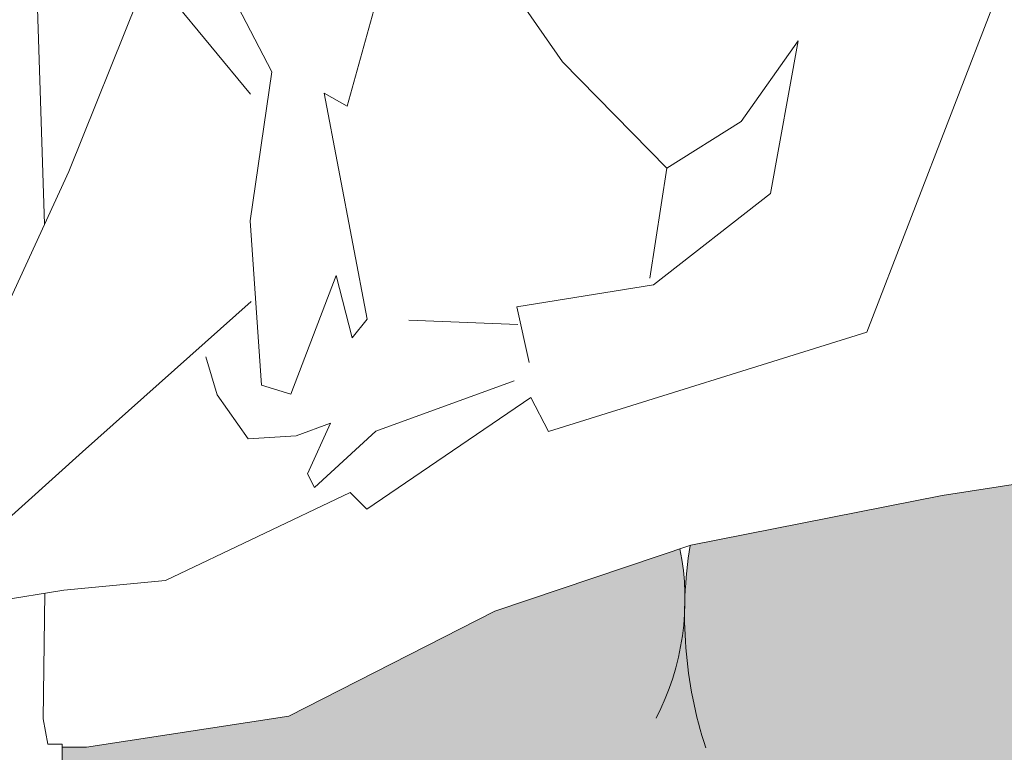
# Model space of a CAD drawing. Units: inches. Extents: x 1994 to 3075, y 3517 to 3950.
# Tile 35 of 58: x 1994.62882 to 1994.65094, y 3553.72103 to 3553.7375. Entities that reach past the tile are written whole.
import ezdxf

# ---------------------------------------------------------------- set-up
doc = ezdxf.new("R2010")
doc.units = ezdxf.units.IN
doc.layers.add('A-FURN-REFR', color=8, linetype='Continuous', lineweight=13)
doc.layers.add('A-FURN-REFR-PATT', color=8, linetype='Continuous', lineweight=13)

msp = doc.modelspace()

# ---------------------------------------------------------------- hatches: boundary and pattern name
at = {"layer": 'A-FURN-REFR-PATT'}
h = msp.add_hatch(color=256, dxfattribs=at)
h.set_gradient(color1=(238, 215, 180), color2=(243, 226, 201), one_color=1, tint=0.87)
edge = h.paths.add_edge_path()
edge.add_line((1994.681542, 3553.709525), (1994.682048, 3553.709217))
edge.add_line((1994.682048, 3553.709217), (1994.682631, 3553.708815))
edge.add_line((1994.682631, 3553.708815), (1994.682631, 3553.708383))
edge.add_line((1994.682631, 3553.708383), (1994.682498, 3553.704652))
edge.add_line((1994.682498, 3553.704652), (1994.682631, 3553.701474))
edge.add_line((1994.682631, 3553.701474), (1994.682631, 3553.700426))
edge.add_line((1994.682631, 3553.700426), (1994.682104, 3553.700396))
edge.add_line((1994.682104, 3553.700396), (1994.681598, 3553.699902))
edge.add_line((1994.681598, 3553.699902), (1994.681992, 3553.699717))
edge.add_line((1994.681992, 3553.699717), (1994.682631, 3553.699439))
edge.add_line((1994.682631, 3553.699439), (1994.682631, 3553.695334))
edge.add_ellipse((1994.680709, 3553.695334), major_axis=(0, 0.002111), ratio=0.910403, start_angle=180, end_angle=270, ccw=False)
edge.add_line((1994.680709, 3553.693223), (1994.680522, 3553.693223))
edge.add_line((1994.680522, 3553.693223), (1994.680314, 3553.694))
edge.add_ellipse((1994.68491, 3553.694998), major_axis=(0, 0.005146), ratio=0.910403, start_angle=92.3431, end_angle=102.2543, ccw=False)
edge.add_ellipse((1994.674568, 3553.694683), major_axis=(0, 0.006219), ratio=0.910403, start_angle=-88.7485, end_angle=-87.76)
edge.add_ellipse((1994.68491, 3553.694998), major_axis=(0, 0.005146), ratio=0.910403, start_angle=91.1484, end_angle=92.3431)
edge.add_ellipse((1994.674568, 3553.694683), major_axis=(0, 0.006219), ratio=0.910403, start_angle=262.8125, end_angle=271.2515, ccw=False)
edge.add_line((1994.680193, 3553.693973), (1994.679278, 3553.693223))
edge.add_line((1994.679278, 3553.693223), (1994.678042, 3553.693223))
edge.add_line((1994.678042, 3553.693223), (1994.673955, 3553.693055))
edge.add_line((1994.673955, 3553.693055), (1994.669892, 3553.693223))
edge.add_line((1994.669892, 3553.693223), (1994.669387, 3553.693223))
edge.add_line((1994.669387, 3553.693223), (1994.668536, 3553.693813))
edge.add_ellipse((1994.673095, 3553.694999), major_axis=(0, 0.005146), ratio=0.910403, start_angle=92.3431, end_angle=104.5922, ccw=False)
edge.add_ellipse((1994.662753, 3553.694684), major_axis=(0, 0.006219), ratio=0.910403, start_angle=-88.7485, end_angle=-87.76)
edge.add_ellipse((1994.673095, 3553.694999), major_axis=(0, 0.005146), ratio=0.910403, start_angle=91.1484, end_angle=92.3431)
edge.add_ellipse((1994.662753, 3553.694684), major_axis=(0, 0.006219), ratio=0.910403, start_angle=260.6759, end_angle=271.2515, ccw=False)
edge.add_line((1994.668352, 3553.693765), (1994.66822, 3553.693223))
edge.add_line((1994.66822, 3553.693223), (1994.666295, 3553.693223))
edge.add_line((1994.666295, 3553.693223), (1994.664702, 3553.693298))
edge.add_line((1994.664702, 3553.693298), (1994.660712, 3553.693051))
edge.add_line((1994.660712, 3553.693051), (1994.65764, 3553.693223))
edge.add_line((1994.65764, 3553.693223), (1994.656797, 3553.693223))
edge.add_line((1994.656797, 3553.693223), (1994.656116, 3553.693819))
edge.add_ellipse((1994.660616, 3553.695249), major_axis=(0, 0.005146), ratio=0.910403, start_angle=92.3431, end_angle=107.6246, ccw=False)
edge.add_ellipse((1994.650274, 3553.694934), major_axis=(0, 0.006219), ratio=0.910403, start_angle=-88.7485, end_angle=-87.76)
edge.add_ellipse((1994.660616, 3553.695249), major_axis=(0, 0.005146), ratio=0.910403, start_angle=91.1484, end_angle=92.3431)
edge.add_ellipse((1994.650274, 3553.694934), major_axis=(0, 0.006219), ratio=0.910403, start_angle=257.752, end_angle=271.2515, ccw=False)
edge.add_line((1994.655829, 3553.693728), (1994.654998, 3553.693223))
edge.add_line((1994.654998, 3553.693223), (1994.649752, 3553.692989))
edge.add_line((1994.649752, 3553.692989), (1994.644994, 3553.693223))
edge.add_line((1994.644994, 3553.693223), (1994.643952, 3553.693223))
edge.add_ellipse((1994.651853, 3553.695067), major_axis=(0, 0.008872), ratio=0.910403, start_angle=89.8354, end_angle=103.1369, ccw=False)
edge.add_ellipse((1994.638929, 3553.695405), major_axis=(0, 0.005332), ratio=0.910403, start_angle=266.2788, end_angle=270.7223)
edge.add_ellipse((1994.651853, 3553.695067), major_axis=(0, 0.008872), ratio=0.910403, start_angle=87.1651, end_angle=89.8354)
edge.add_ellipse((1994.638929, 3553.695405), major_axis=(0, 0.005332), ratio=0.910403, start_angle=243.7698, end_angle=266.2788, ccw=False)
edge.add_line((1994.643359, 3553.693223), (1994.642545, 3553.693223))
edge.add_line((1994.642545, 3553.693223), (1994.641153, 3553.693113))
edge.add_line((1994.641153, 3553.693113), (1994.636432, 3553.693359))
edge.add_line((1994.636432, 3553.693359), (1994.633777, 3553.693223))
edge.add_line((1994.633777, 3553.693223), (1994.63245, 3553.693223))
edge.add_line((1994.63245, 3553.693223), (1994.632375, 3553.693314))
edge.add_ellipse((1994.640193, 3553.695548), major_axis=(0, 0.008872), ratio=0.910403, start_angle=89.8354, end_angle=105.9456, ccw=False)
edge.add_ellipse((1994.627269, 3553.695886), major_axis=(0, 0.005332), ratio=0.910403, start_angle=266.2788, end_angle=270.7223)
edge.add_ellipse((1994.640193, 3553.695548), major_axis=(0, 0.008872), ratio=0.910403, start_angle=87.1651, end_angle=89.8354)
edge.add_ellipse((1994.627269, 3553.695886), major_axis=(0, 0.005332), ratio=0.910403, start_angle=237.8324, end_angle=266.2788, ccw=False)
edge.add_ellipse((1994.6317, 3553.695334), major_axis=(0, 0.002111), ratio=0.910403, start_angle=90, end_angle=174.0631, ccw=False)
edge.add_line((1994.629778, 3553.695334), (1994.629737, 3553.696763))
edge.add_line((1994.629737, 3553.696763), (1994.629778, 3553.698454))
edge.add_line((1994.629778, 3553.698454), (1994.629778, 3553.699441))
edge.add_line((1994.629778, 3553.699441), (1994.629962, 3553.700094))
edge.add_line((1994.629962, 3553.700094), (1994.630637, 3553.700403))
edge.add_line((1994.630637, 3553.700403), (1994.630075, 3553.700834))
edge.add_line((1994.630075, 3553.700834), (1994.629778, 3553.701292))
edge.add_line((1994.629778, 3553.701292), (1994.629778, 3553.702155))
edge.add_line((1994.629778, 3553.702155), (1994.630018, 3553.703363))
edge.add_line((1994.630018, 3553.703363), (1994.630018, 3553.706016))
edge.add_line((1994.630018, 3553.706016), (1994.629778, 3553.708015))
edge.add_line((1994.629778, 3553.708015), (1994.629778, 3553.70894))
edge.add_line((1994.629778, 3553.70894), (1994.630187, 3553.709347))
edge.add_line((1994.630187, 3553.709347), (1994.630918, 3553.70947))
edge.add_line((1994.630918, 3553.70947), (1994.630299, 3553.709902))
edge.add_line((1994.630299, 3553.709902), (1994.629778, 3553.710112))
edge.add_line((1994.629778, 3553.710112), (1994.629778, 3553.712086))
edge.add_line((1994.629778, 3553.712086), (1994.629962, 3553.713788))
edge.add_line((1994.629962, 3553.713788), (1994.629778, 3553.716158))
edge.add_line((1994.629778, 3553.716158), (1994.629778, 3553.718502))
edge.add_line((1994.629778, 3553.718502), (1994.630187, 3553.718908))
edge.add_line((1994.630187, 3553.718908), (1994.629778, 3553.719365))
edge.add_line((1994.629778, 3553.719365), (1994.629778, 3553.72115))
edge.add_line((1994.629778, 3553.72115), (1994.630322, 3553.72115))
edge.add_line((1994.630322, 3553.72115), (1994.634865, 3553.721849))
edge.add_line((1994.634865, 3553.721849), (1994.639494, 3553.724204))
edge.add_line((1994.639494, 3553.724204), (1994.643653, 3553.725608))
edge.add_ellipse((1994.63891, 3553.72447), major_axis=(0, 0.005332), ratio=0.910403, start_angle=270.7223, end_angle=283.4893, ccw=False)
edge.add_ellipse((1994.651833, 3553.724132), major_axis=(0, 0.008872), ratio=0.910403, start_angle=87.1651, end_angle=89.8354)
edge.add_ellipse((1994.63891, 3553.72447), major_axis=(0, 0.005332), ratio=0.910403, start_angle=266.2788, end_angle=270.7223)
edge.add_ellipse((1994.651833, 3553.724132), major_axis=(0, 0.008872), ratio=0.910403, start_angle=438.9501, end_angle=447.1651, ccw=False)
edge.add_line((1994.643881, 3553.725685), (1994.643897, 3553.72569))
edge.add_line((1994.643897, 3553.72569), (1994.649542, 3553.726806))
edge.add_line((1994.649542, 3553.726806), (1994.655977, 3553.727797))
edge.add_line((1994.655977, 3553.727797), (1994.658348, 3553.728382))
edge.add_ellipse((1994.662052, 3553.754177), major_axis=(0, 0.026115), ratio=0.910403, start_angle=171.8281, end_angle=180.2609)
edge.add_ellipse((1994.661314, 3553.682223), major_axis=(0, 0.04585), ratio=0.910403, start_angle=-1.0711, end_angle=-0.1044)
edge.add_ellipse((1994.662052, 3553.754177), major_axis=(0, 0.026115), ratio=0.910403, start_angle=171.8281, end_angle=178.5636, ccw=False)
edge.add_line((1994.658348, 3553.728382), (1994.666025, 3553.730275))
edge.add_line((1994.666025, 3553.730275), (1994.67483, 3553.732877))
edge.add_line((1994.67483, 3553.732877), (1994.680219, 3553.734687))
edge.add_ellipse((1994.675489, 3553.733489), major_axis=(0, 0.005332), ratio=0.910403, start_angle=270.7223, end_angle=284.2178, ccw=False)
edge.add_ellipse((1994.688412, 3553.73315), major_axis=(0, 0.008872), ratio=0.910403, start_angle=87.1651, end_angle=89.8354)
edge.add_ellipse((1994.675489, 3553.733489), major_axis=(0, 0.005332), ratio=0.910403, start_angle=266.2788, end_angle=270.7223)
edge.add_ellipse((1994.688412, 3553.73315), major_axis=(0, 0.008872), ratio=0.910403, start_angle=438.5005, end_angle=447.1651, ccw=False)
edge.add_line((1994.68047, 3553.734766), (1994.682205, 3553.735263))
edge.add_line((1994.682205, 3553.735263), (1994.682631, 3553.735263))
edge.add_line((1994.682631, 3553.735263), (1994.682631, 3553.734609))
edge.add_line((1994.682631, 3553.734609), (1994.682783, 3553.733623))
edge.add_line((1994.682783, 3553.733623), (1994.682631, 3553.730537))
edge.add_line((1994.682631, 3553.730537), (1994.682631, 3553.728749))
edge.add_line((1994.682631, 3553.728749), (1994.682334, 3553.728195))
edge.add_line((1994.682334, 3553.728195), (1994.681547, 3553.727824))
edge.add_line((1994.681547, 3553.727824), (1994.682053, 3553.727639))
edge.add_line((1994.682053, 3553.727639), (1994.682631, 3553.72733))
edge.add_line((1994.682631, 3553.72733), (1994.682631, 3553.725726))
edge.add_line((1994.682631, 3553.725726), (1994.682727, 3553.724308))
edge.add_line((1994.682727, 3553.724308), (1994.682631, 3553.721716))
edge.add_line((1994.682631, 3553.721716), (1994.682631, 3553.720165))
edge.add_line((1994.682631, 3553.720165), (1994.682329, 3553.719086))
edge.add_line((1994.682329, 3553.719086), (1994.681823, 3553.718654))
edge.add_line((1994.681823, 3553.718654), (1994.682329, 3553.718531))
edge.add_line((1994.682329, 3553.718531), (1994.682722, 3553.718346))
edge.add_line((1994.682722, 3553.718346), (1994.68261, 3553.715693))
edge.add_line((1994.68261, 3553.715693), (1994.682631, 3553.711159))
edge.add_line((1994.682631, 3553.711159), (1994.682631, 3553.710327))
edge.add_line((1994.682631, 3553.710327), (1994.682217, 3553.70971))
edge.add_line((1994.682217, 3553.70971), (1994.681542, 3553.709525))
edge = h.paths.add_edge_path(flags=16)
edge.add_ellipse((1994.674017, 3553.663488), major_axis=(0, 0.04585), ratio=0.910403, start_angle=-1.0711, end_angle=-0.1044)
edge.add_ellipse((1994.674755, 3553.735442), major_axis=(0, 0.026115), ratio=0.910403, start_angle=178.5636, end_angle=180.2609)
h.paths.add_polyline_path([(1994.668419, 3553.710039), (1994.668385, 3553.710026), (1994.668404, 3553.710013)], flags=16)
edge = h.paths.add_edge_path(flags=16)
edge.add_ellipse((1994.663397, 3553.714852), major_axis=(0, 0.005332), ratio=0.910403, start_angle=266.2788, end_angle=270.7223)
edge.add_ellipse((1994.67632, 3553.714514), major_axis=(0, 0.008872), ratio=0.910403, start_angle=87.1651, end_angle=89.8354)
edge = h.paths.add_edge_path(flags=16)
edge.add_ellipse((1994.662753, 3553.703926), major_axis=(0, 0.006219), ratio=0.910403, start_angle=-88.7485, end_angle=-87.76)
edge.add_ellipse((1994.673095, 3553.704241), major_axis=(0, 0.005146), ratio=0.910403, start_angle=91.1484, end_angle=92.3431)
h.paths.add_polyline_path([(1994.680357, 3553.710026), (1994.680376, 3553.710013), (1994.680391, 3553.710039)], flags=16)
edge = h.paths.add_edge_path(flags=16)
edge.add_ellipse((1994.684791, 3553.713857), major_axis=(0, 0.005146), ratio=0.910403, start_angle=91.1484, end_angle=92.3431)
edge.add_ellipse((1994.67445, 3553.713542), major_axis=(0, 0.006219), ratio=0.910403, start_angle=-88.7485, end_angle=-87.76)
h.paths.add_polyline_path([(1994.668404, 3553.719229), (1994.668419, 3553.719256), (1994.668385, 3553.719242)], flags=16)
edge = h.paths.add_edge_path(flags=16)
edge.add_ellipse((1994.68491, 3553.704625), major_axis=(0, 0.005146), ratio=0.910403, start_angle=91.1484, end_angle=92.3431)
edge.add_ellipse((1994.674568, 3553.70431), major_axis=(0, 0.006219), ratio=0.910403, start_angle=-88.7485, end_angle=-87.76)
edge = h.paths.add_edge_path(flags=16)
edge.add_ellipse((1994.662353, 3553.744655), major_axis=(0, 0.026115), ratio=0.910403, start_angle=178.5636, end_angle=180.2609)
edge.add_ellipse((1994.661615, 3553.6727), major_axis=(0, 0.04585), ratio=0.910403, start_angle=-1.0711, end_angle=-0.1044)
edge = h.paths.add_edge_path(flags=16)
edge.add_ellipse((1994.662621, 3553.722979), major_axis=(0, 0.006219), ratio=0.910403, start_angle=-88.7485, end_angle=-87.76)
edge.add_ellipse((1994.672963, 3553.723294), major_axis=(0, 0.005146), ratio=0.910403, start_angle=91.1484, end_angle=92.3431)
h.paths.add_polyline_path([(1994.68017, 3553.719242), (1994.680189, 3553.719229), (1994.680204, 3553.719256)], flags=16)
h.paths.add_polyline_path([(1994.668419, 3553.70036), (1994.668385, 3553.700347), (1994.668404, 3553.700334)], flags=16)
edge = h.paths.add_edge_path(flags=16)
edge.add_ellipse((1994.673942, 3553.654177), major_axis=(0, 0.04585), ratio=0.910403, start_angle=-1.0711, end_angle=-0.1044)
edge.add_ellipse((1994.67468, 3553.726132), major_axis=(0, 0.026115), ratio=0.910403, start_angle=178.5636, end_angle=180.2609)
edge = h.paths.add_edge_path(flags=16)
edge.add_ellipse((1994.685026, 3553.723294), major_axis=(0, 0.005146), ratio=0.910403, start_angle=91.1484, end_angle=92.3431)
edge.add_ellipse((1994.674684, 3553.722979), major_axis=(0, 0.006219), ratio=0.910403, start_angle=-88.7485, end_angle=-87.76)
h.paths.add_polyline_path([(1994.680569, 3553.70036), (1994.680535, 3553.700347), (1994.680554, 3553.700334)], flags=16)
h.paths.add_polyline_path([(1994.656068, 3553.710085), (1994.656034, 3553.710071), (1994.656052, 3553.710058)], flags=16)
h.paths.add_polyline_path([(1994.668404, 3553.728426), (1994.668419, 3553.728453), (1994.668385, 3553.728439)], flags=16)
edge = h.paths.add_edge_path(flags=16)
edge.add_ellipse((1994.650317, 3553.713896), major_axis=(0, 0.006219), ratio=0.910403, start_angle=-88.7485, end_angle=-87.76)
edge.add_ellipse((1994.660659, 3553.714211), major_axis=(0, 0.005146), ratio=0.910403, start_angle=91.1484, end_angle=92.3431)
edge = h.paths.add_edge_path(flags=16)
edge.add_ellipse((1994.650274, 3553.70431), major_axis=(0, 0.006219), ratio=0.910403, start_angle=-88.7485, end_angle=-87.76)
edge.add_ellipse((1994.660616, 3553.704625), major_axis=(0, 0.005146), ratio=0.910403, start_angle=91.1484, end_angle=92.3431)
h.paths.add_polyline_path([(1994.68033, 3553.728439), (1994.680349, 3553.728426), (1994.680364, 3553.728453)], flags=16)
h.paths.add_polyline_path([(1994.656052, 3553.719229), (1994.656068, 3553.719256), (1994.656034, 3553.719242)], flags=16)
edge = h.paths.add_edge_path(flags=16)
edge.add_ellipse((1994.649569, 3553.663672), major_axis=(0, 0.04585), ratio=0.910403, start_angle=-1.0711, end_angle=-0.1044)
edge.add_ellipse((1994.650307, 3553.735627), major_axis=(0, 0.026115), ratio=0.910403, start_angle=178.5636, end_angle=180.2609)
h.paths.add_polyline_path([(1994.656068, 3553.700324), (1994.656034, 3553.70031), (1994.656052, 3553.700297)], flags=16)
edge = h.paths.add_edge_path(flags=16)
edge.add_ellipse((1994.650446, 3553.723545), major_axis=(0, 0.006219), ratio=0.910403, start_angle=-88.7485, end_angle=-87.76)
edge.add_ellipse((1994.660788, 3553.72386), major_axis=(0, 0.005146), ratio=0.910403, start_angle=91.1484, end_angle=92.3431)
edge = h.paths.add_edge_path(flags=16)
edge.add_ellipse((1994.64966, 3553.654177), major_axis=(0, 0.04585), ratio=0.910403, start_angle=-1.0711, end_angle=-0.1044)
edge.add_ellipse((1994.650398, 3553.726132), major_axis=(0, 0.026115), ratio=0.910403, start_angle=178.5636, end_angle=180.2609)
h.paths.add_polyline_path([(1994.643774, 3553.710039), (1994.64374, 3553.710026), (1994.643759, 3553.710013)], flags=16)
edge = h.paths.add_edge_path(flags=16)
edge.add_ellipse((1994.638006, 3553.713542), major_axis=(0, 0.006219), ratio=0.910403, start_angle=-88.7485, end_angle=-87.76)
edge.add_ellipse((1994.648347, 3553.713857), major_axis=(0, 0.005146), ratio=0.910403, start_angle=91.1484, end_angle=92.3431)
edge = h.paths.add_edge_path(flags=16)
edge.add_ellipse((1994.638929, 3553.705498), major_axis=(0, 0.005332), ratio=0.910403, start_angle=266.2788, end_angle=270.7223)
edge.add_ellipse((1994.651853, 3553.705159), major_axis=(0, 0.008872), ratio=0.910403, start_angle=87.1651, end_angle=89.8354)
h.paths.add_polyline_path([(1994.643759, 3553.719229), (1994.643774, 3553.719256), (1994.64374, 3553.719242)], flags=16)
h.paths.add_polyline_path([(1994.643774, 3553.700752), (1994.64374, 3553.700739), (1994.643759, 3553.700726)], flags=16)
edge = h.paths.add_edge_path(flags=16)
edge.add_ellipse((1994.637078, 3553.672998), major_axis=(0, 0.04585), ratio=0.910403, start_angle=-1.0711, end_angle=-0.1044)
edge.add_ellipse((1994.637816, 3553.744953), major_axis=(0, 0.026115), ratio=0.910403, start_angle=178.5636, end_angle=180.2609)
edge = h.paths.add_edge_path(flags=16)
edge.add_ellipse((1994.637265, 3553.654177), major_axis=(0, 0.04585), ratio=0.910403, start_angle=-1.0711, end_angle=-0.1044)
edge.add_ellipse((1994.638003, 3553.726132), major_axis=(0, 0.026115), ratio=0.910403, start_angle=178.5636, end_angle=180.2609)
h.paths.add_polyline_path([(1994.632201, 3553.710039), (1994.632167, 3553.710026), (1994.632186, 3553.710013)], flags=16)
edge = h.paths.add_edge_path(flags=16)
edge.add_ellipse((1994.626452, 3553.713542), major_axis=(0, 0.006219), ratio=0.910403, start_angle=-88.7485, end_angle=-87.76)
edge.add_ellipse((1994.636794, 3553.713857), major_axis=(0, 0.005146), ratio=0.910403, start_angle=91.1484, end_angle=92.3431)
edge = h.paths.add_edge_path(flags=16)
edge.add_ellipse((1994.627269, 3553.705498), major_axis=(0, 0.005332), ratio=0.910403, start_angle=266.2788, end_angle=270.7223)
edge.add_ellipse((1994.640193, 3553.705159), major_axis=(0, 0.008872), ratio=0.910403, start_angle=87.1651, end_angle=89.8354)
h.paths.add_polyline_path([(1994.631818, 3553.719229), (1994.631834, 3553.719256), (1994.631799, 3553.719242)], flags=16)
h.paths.add_polyline_path([(1994.631864, 3553.700752), (1994.63183, 3553.700739), (1994.631849, 3553.700726)], flags=16)

# ---------------------------------------------------------------- linework, layer by layer
at = {"layer": 'A-FURN-REFR'}
for p, q in [((1994.638071, 3553.740802), (1994.641011, 3553.736552)), ((1994.637273, 3553.739491), (1994.636173, 3553.735557)), ((1994.629193, 3553.738583), (1994.629381, 3553.732902)), ((1994.629921, 3553.734084), (1994.631778, 3553.738695)), ((1994.632016, 3553.738235), (1994.634003, 3553.735824)), ((1994.650846, 3553.738236), (1994.64785, 3553.730478)), ((1994.634482, 3553.736326), (1994.633608, 3553.738012)), ((1994.64503, 3553.735209), (1994.646306, 3553.737021)), ((1994.646306, 3553.737021), (1994.645685, 3553.733589)), ((1994.641011, 3553.736552), (1994.643357, 3553.734163)), ((1994.634, 3553.732981), (1994.634482, 3553.736326)), ((1994.635656, 3553.735843), (1994.636624, 3553.730766)), ((1994.636173, 3553.735557), (1994.635656, 3553.735843)), ((1994.643357, 3553.734163), (1994.64503, 3553.735209)), ((1994.643357, 3553.734163), (1994.642975, 3553.731692)), ((1994.628623, 3553.731244), (1994.629921, 3553.734084)), ((1994.645685, 3553.733589), (1994.643055, 3553.731539)), ((1994.634254, 3553.729284), (1994.634, 3553.732981)), ((1994.635929, 3553.731752), (1994.63491, 3553.729086)), ((1994.636285, 3553.730351), (1994.635929, 3553.731752)), ((1994.643055, 3553.731539), (1994.639989, 3553.731043)), ((1994.634017, 3553.731166), (1994.630231, 3553.727784)), ((1994.639989, 3553.731043), (1994.640266, 3553.729796)), ((1994.636624, 3553.730766), (1994.636285, 3553.730351)), ((1994.640008, 3553.730649), (1994.63756, 3553.730742)), ((1994.64785, 3553.730478), (1994.640701, 3553.728242)), ((1994.633, 3553.729921), (1994.633258, 3553.729068)), ((1994.63491, 3553.729086), (1994.634254, 3553.729284)), ((1994.63682, 3553.72825), (1994.639927, 3553.729381)), ((1994.633258, 3553.729068), (1994.633953, 3553.728082)), ((1994.640304, 3553.729008), (1994.636619, 3553.726501)), ((1994.640701, 3553.728242), (1994.640304, 3553.729008)), ((1994.635028, 3553.728145), (1994.635805, 3553.728428)), ((1994.635805, 3553.728428), (1994.635286, 3553.727292)), ((1994.635445, 3553.726985), (1994.63682, 3553.72825)), ((1994.633953, 3553.728082), (1994.635028, 3553.728145)), ((1994.630231, 3553.727784), (1994.625947, 3553.723933)), ((1994.649542, 3553.726806), (1994.655977, 3553.727797)), ((1994.635286, 3553.727292), (1994.635445, 3553.726985)), ((1994.636241, 3553.726874), (1994.632098, 3553.724893)), ((1994.636619, 3553.726501), (1994.636241, 3553.726874)), ((1994.643897, 3553.72569), (1994.649542, 3553.726806)), ((1994.639494, 3553.724204), (1994.643897, 3553.72569)), ((1994.632098, 3553.724893), (1994.629809, 3553.724679)), ((1994.629809, 3553.724679), (1994.626743, 3553.724183)), ((1994.629384, 3553.724611), (1994.629351, 3553.72179)), ((1994.634865, 3553.721849), (1994.639494, 3553.724204)), ((1994.629351, 3553.72179), (1994.629455, 3553.721215)), ((1994.630322, 3553.72115), (1994.634865, 3553.721849)), ((1994.629455, 3553.721215), (1994.629778, 3553.721215)), ((1994.629778, 3553.719365), (1994.629778, 3553.721215)), ((1994.630322, 3553.72115), (1994.629778, 3553.72115))]:
    msp.add_line(p, q, dxfattribs=at)
at = {"layer": 'A-FURN-REFR', "extrusion": (0, 0, -1)}
for centre, major_axis, start_param, end_param in [((1994.63891, 3553.72447), (0, 0.005332), 1.355783, 2.094288), ((1994.651833, 3553.724132), (0, 0.008872), 4.368048, 4.888339)]:
    msp.add_ellipse(centre, major_axis=major_axis, ratio=0.910403, start_param=start_param, end_param=end_param, dxfattribs=at)

doc.saveas('drawing.dxf')
